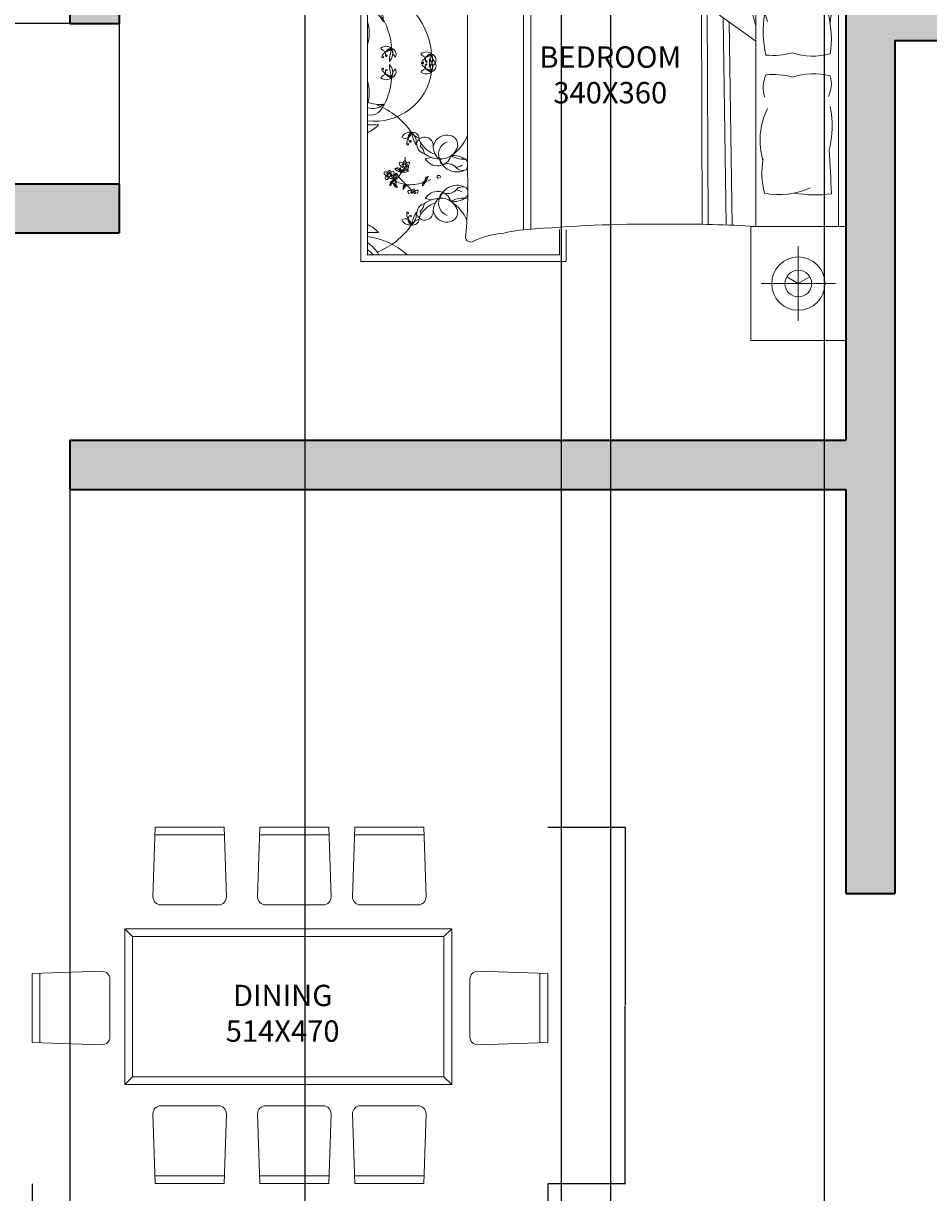
# Model space of a CAD drawing. Units: centimetres. Extents: x 2178 to 3635, y 1064 to 2635.
# Tile 6 of 9: x 2788 to 3211, y 1765 to 2312. Entities that reach past the tile are written whole.
import ezdxf

# ---------------------------------------------------------------- set-up
doc = ezdxf.new("R2010")
doc.units = ezdxf.units.CM
for name, color, linetype, lineweight in [('A-ANNO-DIMS', 2, 'Continuous', 18), ('A-AREA-IDEN', 7, 'Continuous', 18), ('A-DOOR', 32, 'Continuous', 25), ('A-FURN', 42, 'Continuous', 18), ('A-WALL', 7, 'Continuous', 35)]:
    doc.layers.add(name, color=color, linetype=linetype, lineweight=lineweight)
doc.layers.add('A-WALL-PATT', color=18, linetype='Continuous', lineweight=13, true_color=0x000000)
doc.styles.get("Standard").update_dxf_attribs({"font": 'arial.ttf'})
doc.dimstyles.get("Standard").update_dxf_attribs({"dimtxt": 0.18, "dimasz": 0.18, "dimexe": 0.18, "dimexo": 0.0625, "dimgap": 0.09, "dimtad": 0, "dimtih": 1, "dimtoh": 1, "dimdec": 4, "dimzin": 0, "dimdsep": 46, "dimtxsty": 'Standard', "dimcen": 0.09, "dimadec": 0, "dimazin": 0, "dimtfac": 1, "dimtdec": 4, "dimtofl": 0, "dimtmove": 0, "dimatfit": 3, "dimfxl": 1, "dimtolj": 1, "dimtzin": 0, "dimarcsym": 0})

# ---------------------------------------------------------------- blocks, each defined once
blk = doc.blocks.new('bed')
for p, q in [((2798.77, 2937.13), (3098.77, 2937.13)), ((2858.77, 2937.13), (2858.77, 2854.79)), ((2828.77, 2892.53), (2828.77, 2931.73)), ((3038.77, 2933.28), (2858.77, 2933.28)), ((3068.77, 2892.53), (3068.77, 2931.73)), ((2848.37, 2912.13), (2809.17, 2912.13)), ((3049.17, 2912.13), (3088.37, 2912.13)), ((2858.77, 2889.72), (3038.77, 2889.72)), ((2900.44, 2880.8), (2933.16, 2889.72)), ((2941.19, 2889.72), (2924.75, 2866.84)), ((2878.57, 2872.91), (2900.44, 2880.8)), ((2867.02, 2864.41), (2878.57, 2872.91)), ((3037.85, 2874.18), (2928.92, 2872.64)), ((3037.97, 2877.26), (2931.16, 2875.76)), ((2924.75, 2866.84), (2918.06, 2849.23)), ((2856.09, 2851.66), (2867.02, 2864.41)), ((3037.71, 2861.65), (2922.6, 2861.18)), ((3037.69, 2864.73), (2923.78, 2864.28)), ((2858.52, 2849.23), (2856.09, 2851.66)), ((2870.67, 2850.44), (2858.52, 2849.23)), ((2885.86, 2849.23), (2870.67, 2850.44)), ((2899.23, 2847.41), (2885.86, 2849.23)), ((2907.13, 2843.76), (2899.23, 2847.41)), ((2918.06, 2849.23), (2916.85, 2841.33)), ((2916.85, 2841.33), (2907.13, 2843.76)), ((2838.37, 2790.07), (2855.34, 2790.07)), ((2838.37, 2682), (2838.37, 2790.07)), ((2855.33, 2786.59), (2841.85, 2786.59)), ((2841.85, 2786.59), (2841.85, 2685.48)), ((3053.6, 2786.59), (3040.38, 2786.59)), ((3040.44, 2790.07), (3057.08, 2790.07)), ((3053.6, 2685.48), (3053.6, 2786.59)), ((3057.08, 2790.07), (3057.08, 2682)), ((3040.42, 2767.62), (2855.31, 2767.62)), ((3040.13, 2771.36), (2855.32, 2771.36)), ((3009.67, 2738.15), (2887.87, 2738.15)), ((2871.41, 2715.89), (2870.75, 2719.28)), ((2892.38, 2715.89), (2893.04, 2719.28)), ((3003.07, 2715.89), (3002.41, 2719.28)), ((3024.04, 2715.89), (3024.7, 2719.28)), ((3057.08, 2682), (2838.37, 2682)), ((2841.85, 2685.48), (3053.6, 2685.48))]:
    blk.add_line(p, q)
for points in [[(2858.77, 2887.13), (2798.77, 2887.13), (2798.77, 2937.13)], [(3038.77, 2937.13), (3038.77, 2887.13), (3098.77, 2887.13), (3098.77, 2937.13)], [(2828.77, 2912.13), (2832.27, 2918.19)], [(3068.77, 2912.13), (3065.27, 2918.19)], [(2828.77, 2912.13), (2832.27, 2906.07)], [(3068.77, 2912.13), (3065.27, 2906.07)]]:
    blk.add_lwpolyline(points)
for points in [[(2876, 2929.65, 0.074897), (2876.37, 2910.06, -0.472817)], [(2947.37, 2908.96, 0.14099), (2947.97, 2928.95, 0.235245)], [(2960.18, 2908.96, -0.14099), (2959.58, 2928.95, -0.235245)], [(3021.54, 2929.65, -0.074897), (3021.18, 2910.06, 0.472817)], [(2855.46, 2824.19, 0.001242), (2855.31, 2767.26, -0.127202), (2849.3, 2738.9)], [(3040.05, 2773.72, 0.056112), (3042.23, 2757.21, 0.095341), (3046.45, 2741.32)]]:
    blk.add_lwpolyline(points, format="xyb")
for centre, radius in [((2828.77, 2912.13), 14), ((3068.77, 2912.13), 14), ((2828.77, 2912.13), 7), ((3068.77, 2912.13), 7), ((2888.74, 2705.02), 0.764), ((3006.71, 2705.02), 0.764), ((2883.74, 2696.97), 0.764), ((3011.71, 2696.97), 0.764)]:
    blk.add_circle(centre, radius)
for centre, radius, start, end in [((3041.36, 5784.66), 2859.79, 266.68521, 267.14978), ((2917.11, 2821.09), 108.8, 82.21958, 99.49698), ((2940.09, 2876.08), 53.46, 81.52493, 103.95996), ((2963.69, 2914.69), 14.84, 63.34374, 106.10256), ((2985.93, 2877.16), 52.74, 76.34271, 101.1841), ((2856.18, 5784.66), 2859.79, 272.85022, 273.31479), ((2914.22, 2902.19), 38.67, 155.1316, 191.75834), ((2983.32, 2902.19), 38.67, 348.24166, 24.8684), ((2912, 2898.93), 36.76, 354.01289, 15.82928), ((2995.54, 2898.93), 36.76, 164.17072, 185.98711), ((2886.7, 2933.16), 40.2, 255.10393, 281.03689), ((2907.87, 2961.74), 69.73, 258.03974, 289.26152), ((2936.1, 2946.52), 52.9, 259.86169, 283.62376), ((2965.7, 2909.52), 15.9, 245.01826, 288.54073), ((2993.49, 2930.2), 38.19, 243.87611, 286.17464), ((3010.84, 2933.16), 40.2, 258.96311, 284.89607), ((3576.57, 2853.06), 539.05, 176.09997, 180.92818), ((2581.02, 2844.2), 275.17, 355.82941, 1.55305), ((2888.28, 2822.94), 24.42, 66.26158, 101.3392), ((2861.22, 2957.89), 113.22, 267.45188, 281.3392), ((2937.68, 2954.7), 116.34, 250.11942, 259.33829), ((2916.17, 2841.09), 0.724, 268.86235, 19.75363), ((3740.68, 2833.46), 703.17, 179.11454, 184.87351), ((2852.06, 2739.09), 2.77, 183.97998, 297.34124), ((2884.29, 2425.86), 312.3, 89.34325, 95.68869), ((2850.89, 2717.02), 22.71, 33.66712, 63.29966), ((2881.32, 2730.53), 11.57, 145.78505, 184.73037), ((2859.22, 2735.93), 12.43, 328.82178, 9.15542), ((2874.61, 2734.83), 3.61, 120.0293, 142.32497), ((2868.85, 2732.7), 9.56, 289.28218, 29.1751), ((2873.09, 2735.54), 4.49, 311.56531, 23.83541), ((2874.61, 2734.83), 3.61, 44.45169, 63.55801), ((2894.94, 2732.7), 9.56, 150.8249, 250.71782), ((2890.7, 2735.54), 4.49, 156.16459, 228.43469), ((2889.17, 2734.83), 3.61, 113.22901, 135.54831), ((2889.17, 2734.83), 3.61, 37.67503, 66.71436), ((2882.46, 2730.53), 11.57, 355.26963, 34.21495), ((2904.56, 2735.93), 12.43, 169.71335, 211.17822), ((2912.89, 2717.02), 22.71, 111.49413, 146.33288), ((2982.56, 2717.02), 22.71, 33.66712, 68.50587), ((3012.99, 2730.53), 11.57, 145.78505, 184.73037), ((2990.89, 2735.93), 12.43, 328.82178, 10.28665), ((3006.28, 2734.83), 3.61, 113.28564, 142.32497), ((3000.51, 2732.7), 9.56, 289.28218, 29.1751), ((3006.28, 2734.83), 3.61, 44.45169, 66.71436), ((3004.75, 2735.54), 4.49, 311.56531, 23.83541), ((3018.86, 2446.37), 291.92, 85.24024, 91.80351), ((3026.6, 2732.7), 9.56, 150.8249, 250.71782), ((3022.36, 2735.54), 4.49, 156.16459, 228.43469), ((3020.84, 2734.83), 3.61, 106.63434, 135.54831), ((3020.84, 2734.83), 3.61, 37.67503, 72.58143), ((3014.13, 2730.53), 11.57, 355.26963, 34.21495), ((3036.23, 2735.93), 12.43, 169.24899, 211.17822), ((3044.56, 2717.02), 22.71, 113.64533, 146.33288), ((3044.17, 2739.79), 2.73, 246.52186, 33.82642), ((2864.12, 2727.92), 5.07, 84.48557, 181.05378), ((2862.56, 2724.18), 9.02, 355.29334, 76.921), ((2880.15, 2727.58), 6.15, 131.56531, 195.14713), ((2867.4, 2730.97), 8.62, 7.43599, 29.91487), ((2883.64, 2727.58), 6.15, 344.85287, 48.43469), ((2896.38, 2730.97), 8.62, 150.08513, 172.56401), ((2901.22, 2724.18), 9.02, 103.079, 184.70666), ((2899.66, 2727.92), 5.07, 358.94622, 95.51443), ((2995.79, 2727.92), 5.07, 84.48557, 181.05378), ((2994.23, 2724.18), 9.02, 355.29334, 76.921), ((3011.81, 2727.58), 6.15, 131.56531, 195.14713), ((2999.07, 2730.97), 8.62, 7.43599, 29.91487), ((3015.3, 2727.58), 6.15, 344.85287, 48.43469), ((3028.05, 2730.97), 8.62, 150.08513, 172.56401), ((3032.89, 2724.18), 9.02, 103.079, 184.70666), ((3031.33, 2727.92), 5.07, 358.94622, 95.51443), ((2866.2, 2727.2), 7.17, 174.94485, 262.88575), ((2869.01, 2729.92), 6.96, 201.58187, 291.42215), ((2867.69, 2722.36), 7.46, 299.90854, 73.1337), ((2872.41, 2725.49), 1.86, 257.30406, 15.14713), ((2896.09, 2722.36), 7.46, 106.8663, 240.09146), ((2891.37, 2725.49), 1.86, 164.85287, 282.69594), ((2894.77, 2729.92), 6.96, 248.57785, 338.41813), ((2897.59, 2727.2), 7.17, 277.11425, 5.05515), ((2997.86, 2727.2), 7.17, 174.94485, 262.88575), ((3000.68, 2729.92), 6.96, 201.58187, 291.42215), ((2999.36, 2722.36), 7.46, 299.90854, 73.1337), ((3004.08, 2725.49), 1.86, 257.30406, 15.14713), ((3027.76, 2722.36), 7.46, 106.8663, 240.09146), ((3023.04, 2725.49), 1.86, 164.85287, 282.69594), ((3026.44, 2729.92), 6.96, 248.57785, 338.41813), ((3029.25, 2727.2), 7.17, 277.11425, 5.05515), ((2864.55, 2715.65), 4.5, 80.26398, 250.86884), ((2855.62, 2725.56), 14.16, 301.26137, 341.7045), ((2864.95, 2728.79), 8.71, 272.3591, 324.04014), ((2855.49, 2724.42), 16.1, 326.28828, 356.5076), ((2881.32, 2730.53), 11.57, 212.70113, 216.34448), ((2903.55, 2707.57), 24.85, 153.0032, 159.89408), ((2882.75, 2722.67), 0.578, 102.70507, 280.43845), ((2882.69, 2723.02), 0.94, 280.43845, 100.41356), ((2882.46, 2730.53), 11.57, 323.65552, 327.29887), ((2898.83, 2728.79), 8.71, 215.95986, 267.6409), ((2908.3, 2724.42), 16.1, 183.4924, 213.71172), ((2908.16, 2725.56), 14.16, 198.2955, 238.73863), ((2899.24, 2715.65), 4.5, 289.13116, 99.73602), ((2951.1, 2680.2), 39.18, 94.46233, 172.25504), ((2951.27, 2716.33), 4.34, 137.78732, 219.11446), ((2946.34, 2716.47), 3.27, 298.5391, 58.36268), ((2951.26, 2719.13), 3.2, 177.75849, 283.85198), ((2951.17, 2718.35), 3.25, 63.02737, 163.80375), ((2947.89, 2725.94), 6.69, 271.45846, 315.37266), ((2950.61, 2713.61), 6.19, 45.54113, 114.31008), ((2956.25, 2745.4), 27.41, 252.59304, 267.25817), ((2957.43, 2722.47), 9.91, 198.91595, 238.01098), ((2954.84, 2713.61), 6.19, 65.68992, 134.45887), ((2949.2, 2745.4), 27.41, 272.74183, 287.40696), ((2954.28, 2718.35), 3.25, 16.19625, 116.97263), ((2957.56, 2725.94), 6.69, 224.62734, 268.54154), ((2948.02, 2722.47), 9.91, 301.98902, 341.08405), ((2954.19, 2719.13), 3.2, 256.14802, 2.24151), ((2959.11, 2716.47), 3.27, 121.63732, 241.4609), ((2954.18, 2716.33), 4.34, 320.88554, 42.21268), ((2953.08, 2689.24), 30.32, 352.86355, 81.81966), ((2996.21, 2715.65), 4.5, 80.26398, 250.86884), ((2987.29, 2725.56), 14.16, 301.26137, 341.7045), ((2996.62, 2728.79), 8.71, 272.3591, 324.04014), ((2987.15, 2724.42), 16.1, 326.28828, 356.5076), ((3012.99, 2730.53), 11.57, 212.70113, 216.34448), ((3012.76, 2723.02), 0.94, 79.58644, 259.56155), ((3012.7, 2722.67), 0.578, 259.56155, 77.29493), ((2991.9, 2707.57), 24.85, 20.10592, 26.9968), ((3014.13, 2730.53), 11.57, 323.65552, 327.29887), ((3030.5, 2728.79), 8.71, 215.95986, 267.6409), ((3039.96, 2724.42), 16.1, 183.4924, 213.71172), ((3039.83, 2725.56), 14.16, 198.2955, 238.73863), ((3030.9, 2715.65), 4.5, 289.13116, 99.73602), ((2860.73, 2709.42), 3.25, 92.95159, 193.72796), ((2854.09, 2714.37), 6.69, 301.38267, 345.29688), ((2863.62, 2710.77), 2.76, 63.97555, 143.26805), ((2863.47, 2717), 5.62, 265.96902, 344.3045), ((2869.52, 2709.53), 5.99, 96.1662, 141.58255), ((2875.21, 2711.65), 0.59, 345.23556, 144.9248), ((2879.44, 2713.73), 1.58, 101.32561, 154.46214), ((2877.17, 2719.07), 4.74, 280.25878, 300.65599), ((2878.27, 2722.86), 8.46, 268.32639, 277.13024), ((2903.55, 2707.57), 24.85, 163.58418, 183.82768), ((2876.15, 2719.06), 4.82, 308.21012, 316.30712), ((2879.11, 2715.89), 1.44, 278.34322, 4.28685), ((2878.31, 2717.16), 2.51, 300.65599, 332.63414), ((2880.2, 2715.5), 0.611, 55.76575, 157.44165), ((2881.15, 2716.07), 0.611, 84.37838, 186.05427), ((2880.58, 2718.52), 2.51, 269.18588, 301.16403), ((2881.32, 2717.22), 1.44, 237.53317, 323.47681), ((2879.92, 2721.32), 4.82, 285.51291, 293.60991), ((2883.07, 2715.9), 1.58, 87.35788, 140.49441), ((2879.43, 2720.42), 4.74, 301.16403, 321.56124), ((2875.57, 2721.25), 8.46, 324.68979, 333.49364), ((2894.26, 2709.53), 5.99, 38.41745, 83.8338), ((2900.32, 2717), 5.62, 195.6955, 274.03098), ((2900.16, 2710.77), 2.76, 36.73195, 116.02445), ((2903.05, 2709.42), 3.25, 346.27204, 87.04841), ((2909.69, 2714.37), 6.69, 194.70312, 238.61733), ((2951.92, 2716.43), 0.424, 283.85198, 219.92454), ((2952.44, 2714.47), 0.487, 238.01098, 71.55918), ((2952.52, 2714.71), 0.236, 71.55918, 188.01668), ((2953.01, 2714.47), 0.487, 108.44082, 301.98902), ((2952.93, 2714.71), 0.236, 351.98332, 108.44082), ((2953.49, 2716.59), 0.255, 320.19092, 256.02088), ((2992.4, 2709.42), 3.25, 92.95159, 193.72796), ((2985.76, 2714.37), 6.69, 301.38267, 345.29688), ((2995.29, 2710.77), 2.76, 63.97555, 143.26805), ((2995.13, 2717), 5.62, 265.96902, 344.3045), ((3001.19, 2709.53), 5.99, 96.1662, 141.58255), ((3012.38, 2715.9), 1.58, 39.50559, 92.64212), ((3016.02, 2720.42), 4.74, 218.43876, 238.83597), ((3019.88, 2721.25), 8.46, 206.50636, 215.31021), ((3014.13, 2717.22), 1.44, 216.52319, 302.46683), ((3014.87, 2718.52), 2.51, 238.83597, 270.81412), ((3015.53, 2721.32), 4.82, 246.39009, 254.48709), ((3014.3, 2716.07), 0.611, 353.94573, 95.62162), ((3016.34, 2715.89), 1.44, 175.71315, 261.65678), ((3015.25, 2715.5), 0.611, 22.55835, 124.23425), ((3017.14, 2717.16), 2.51, 207.36586, 239.34401), ((2991.9, 2707.57), 24.85, 356.17232, 16.41582), ((3019.3, 2719.06), 4.82, 223.69288, 231.78988), ((3018.28, 2719.07), 4.74, 239.34401, 259.74122), ((3017.18, 2722.86), 8.46, 262.86976, 271.67361), ((3016.01, 2713.73), 1.58, 25.53786, 78.67439), ((3020.24, 2711.65), 0.59, 35.0752, 194.76444), ((3031.98, 2717), 5.62, 195.6955, 274.03098), ((3025.93, 2709.53), 5.99, 38.41745, 83.8338), ((3031.83, 2710.77), 2.76, 36.73195, 116.02445), ((3041.36, 2714.37), 6.69, 194.70312, 238.61733), ((3034.72, 2709.42), 3.25, 346.27204, 87.04841), ((2812.68, 2680.2), 39.18, 7.74496, 41.8856), ((2879.7, 2676.32), 39.18, 124.38655, 158.59079), ((2861.82, 2707.73), 4.34, 167.71153, 249.03868), ((2862.6, 2705.03), 6.19, 75.46535, 144.23429), ((2851.64, 2735.41), 27.41, 282.51726, 297.18239), ((2857.48, 2705.38), 3.27, 328.46331, 88.28689), ((2864.1, 2716.11), 9.91, 228.84017, 267.9352), ((2860.42, 2710.14), 3.2, 207.6827, 313.77619), ((2862.34, 2708.13), 0.424, 313.77619, 249.71835), ((2863.71, 2706.94), 0.236, 101.4834, 217.94089), ((2863.76, 2706.7), 0.487, 267.9352, 101.4834), ((2874.99, 2710.74), 1.27, 101.56373, 142.6358), ((2873.93, 2709.56), 0.764, 273.27684, 86.72316), ((2874.97, 2708.15), 1.26, 217.76209, 259.04026), ((2874.82, 2710.28), 0.73, 91.10805, 181.86747), ((2876.33, 2709.83), 2.32, 203.42757, 227.61037), ((2875.59, 2708.82), 1.58, 80.3487, 133.65382), ((2875.31, 2710.12), 1.25, 229.78892, 317.67915), ((2873.96, 2711.74), 1.84, 288.72627, 352.50315), ((2873.9, 2707.47), 1.78, 355.05304, 68.36176), ((2875.3, 2707.17), 2.5, 83.08516, 105.71709), ((2875.09, 2707.37), 0.586, 232.47371, 355.05304), ((2857.98, 2686.43), 28.48, 43.15413, 52.0459), ((2875.75, 2709.72), 0.658, 317.67915, 80.3487), ((2877.32, 2705.8), 1.44, 278.34322, 4.28685), ((2876.52, 2707.06), 2.51, 300.65599, 332.63414), ((2878.41, 2705.4), 0.611, 55.76575, 157.44165), ((2891.17, 2706.94), 12.46, 184.75602, 209.20408), ((2909.1, 2733.46), 40.99, 222.24124, 232.17444), ((2882.89, 2706.16), 3.48, 304.53686, 16.36991), ((2887.73, 2705.18), 2.46, 127.31045, 187.92519), ((2884.34, 2705.45), 2.53, 355.01064, 41.65801), ((2887.9, 2706.08), 1.04, 126.10456, 271.42811), ((2887.78, 2706.37), 0.749, 353.75256, 131.70535), ((2887.08, 2705.48), 1.05, 0.06451, 61.15075), ((2887.33, 2706.37), 1.2, 311.84125, 355.78771), ((2889.8, 2706.2), 1.27, 101.56373, 176.36503), ((2889.63, 2705.74), 0.73, 91.10805, 181.86747), ((2888.77, 2707.2), 1.84, 288.72627, 352.50315), ((2890.02, 2707.11), 0.59, 345.23556, 144.9248), ((2900.02, 2706.7), 0.487, 78.5166, 272.0648), ((2901.18, 2705.03), 6.19, 35.76571, 104.53465), ((2912.15, 2735.41), 27.41, 242.81761, 257.48274), ((2899.68, 2716.11), 9.91, 272.0648, 311.15983), ((2900.07, 2706.94), 0.236, 322.05911, 78.5166), ((2903.37, 2710.14), 3.2, 226.22381, 332.3173), ((2901.49, 2708.3), 0.255, 290.26671, 226.22708), ((2906.3, 2705.38), 3.27, 91.71311, 211.53669), ((2901.96, 2707.73), 4.34, 290.96132, 12.28847), ((2884.08, 2676.32), 39.18, 21.40921, 55.61345), ((3011.37, 2676.32), 39.18, 124.38655, 158.59079), ((2993.49, 2707.73), 4.34, 167.71153, 249.03868), ((2994.27, 2705.03), 6.19, 75.46535, 144.23429), ((2983.3, 2735.41), 27.41, 282.51726, 297.18239), ((2992.08, 2710.14), 3.2, 207.6827, 313.77619), ((2995.76, 2716.11), 9.91, 228.84017, 267.9352), ((2989.15, 2705.38), 3.27, 328.46331, 88.28689), ((2994.01, 2708.13), 0.424, 313.77619, 249.71835), ((2995.38, 2706.94), 0.236, 101.4834, 217.94089), ((2995.43, 2706.7), 0.487, 267.9352, 101.4834), ((3005.43, 2707.11), 0.59, 35.0752, 194.76444), ((3006.68, 2707.2), 1.84, 187.49685, 251.27373), ((3005.82, 2705.74), 0.73, 358.13253, 88.89195), ((3005.65, 2706.2), 1.27, 3.63497, 78.43627), ((3007.67, 2706.37), 0.749, 48.29465, 186.24744), ((3008.12, 2706.37), 1.2, 184.21229, 228.15875), ((3008.37, 2705.48), 1.05, 118.84925, 179.93549), ((3007.55, 2706.08), 1.04, 268.57189, 53.89544), ((3011.11, 2705.45), 2.53, 138.34199, 184.98936), ((3012.56, 2706.16), 3.48, 163.63009, 235.46314), ((3007.72, 2705.18), 2.46, 352.07481, 52.68955), ((2986.35, 2733.46), 40.99, 307.82556, 317.75876), ((3004.28, 2706.94), 12.46, 330.79592, 355.24398), ((3037.47, 2686.43), 28.48, 127.9541, 136.84587), ((3017.04, 2705.4), 0.611, 22.55835, 124.23425), ((3018.13, 2705.8), 1.44, 175.71315, 261.65678), ((3018.93, 2707.06), 2.51, 207.36586, 239.34401), ((3019.7, 2709.72), 0.658, 99.6513, 222.32085), ((3020.14, 2710.12), 1.25, 222.32085, 310.21108), ((3019.86, 2708.82), 1.58, 46.34618, 99.6513), ((3021.49, 2711.74), 1.84, 187.49685, 251.27373), ((3021.55, 2707.47), 1.78, 111.63824, 184.94696), ((3020.36, 2707.37), 0.586, 184.94696, 307.52629), ((3020.15, 2707.17), 2.5, 74.28291, 96.91484), ((3020.63, 2710.28), 0.73, 358.13253, 88.89195), ((3019.12, 2709.83), 2.32, 312.38963, 336.57243), ((3020.46, 2710.74), 1.27, 37.3642, 78.43627), ((3020.48, 2708.15), 1.26, 280.95974, 322.23791), ((3021.52, 2709.56), 0.764, 93.27684, 266.72316), ((3031.69, 2706.7), 0.487, 78.5166, 272.0648), ((3032.85, 2705.03), 6.19, 35.76571, 104.53465), ((3043.81, 2735.41), 27.41, 242.81761, 257.48274), ((3031.35, 2716.11), 9.91, 272.0648, 311.15983), ((3031.74, 2706.94), 0.236, 322.05911, 78.5166), ((3035.03, 2710.14), 3.2, 226.22381, 332.3173), ((3033.16, 2708.3), 0.255, 290.26671, 226.22708), ((3037.97, 2705.38), 3.27, 91.71311, 211.53669), ((3033.63, 2707.73), 4.34, 290.96132, 12.28847), ((3015.75, 2676.32), 39.18, 21.40921, 55.61345), ((3082.77, 2680.2), 39.18, 138.1144, 172.25504), ((2877.65, 2703.63), 1.58, 101.32561, 154.46214), ((2875.39, 2708.98), 4.74, 280.25878, 300.65599), ((2876.48, 2712.77), 8.46, 268.32639, 277.13024), ((2878.18, 2700.87), 0.853, 146.86359, 236.90213), ((2874.36, 2708.97), 4.82, 308.21012, 316.30712), ((2890.21, 2719.66), 22.32, 235.1882, 238.88441), ((2879.65, 2702.11), 2.31, 199.47987, 267.68284), ((2879.39, 2701.23), 1.99, 212.81548, 277.39917), ((2879.13, 2701.31), 0.883, 238.88441, 314.26458), ((2878.94, 2699.33), 1.99, 280.30568, 17.1958), ((2880.21, 2699.7), 0.666, 19.36054, 201.75478), ((2880.22, 2700.2), 0.666, 311.87034, 134.26458), ((2892.74, 2694.13), 13.31, 153.78194, 158.29129), ((2882.15, 2703.22), 3.48, 247.23048, 319.06353), ((2881, 2702.05), 2.05, 264.45436, 310.61881), ((2891.17, 2706.94), 12.46, 214.00334, 222.49171), ((2882.5, 2701.23), 2.12, 218.32082, 298.81623), ((2892.45, 2690.4), 14.94, 120.54402, 139.81798), ((2883.94, 2698.62), 2.46, 70.00407, 130.61881), ((2882.35, 2701.62), 2.53, 297.70426, 344.35163), ((2884.75, 2705.38), 2.12, 272.84988, 356.12261), ((2883.26, 2704.56), 2.05, 321.76073, 7.92519), ((2883.69, 2701.61), 2.05, 8.72271, 54.88717), ((2883.8, 2699.97), 3.48, 0.278, 72.11105), ((2885.36, 2701.25), 2.12, 20.5253, 88.5375), ((2888.15, 2702.29), 2.46, 188.72271, 249.33746), ((2887.13, 2703.59), 0.757, 148.0499, 225.62681), ((2892.45, 2690.4), 14.94, 113.05007, 113.84774), ((2888.54, 2702.71), 2.41, 104.75581, 148.0499), ((2887.18, 2704.44), 1.51, 247.40857, 351.43859), ((2884.99, 2701.06), 2.53, 334.9899, 21.63727), ((2887.61, 2704.38), 0.506, 262.90601, 7.13198), ((2889.78, 2703.61), 1.26, 151.21959, 259.04026), ((2891.14, 2705.29), 2.32, 203.42757, 227.61037), ((2890.41, 2704.28), 1.58, 80.3487, 133.65382), ((2890.12, 2705.58), 1.25, 229.78892, 317.67915), ((2888.71, 2702.93), 1.78, 355.05304, 68.36176), ((2890.11, 2702.63), 2.5, 83.08516, 105.71709), ((2889.9, 2702.83), 0.586, 232.47371, 355.05304), ((2890.56, 2705.18), 0.658, 317.67915, 80.3487), ((2892.45, 2690.4), 14.94, 87.10709, 94.75853), ((2948.18, 2697.36), 3.25, 63.02737, 163.80375), ((2944.89, 2704.96), 6.69, 271.45846, 315.37266), ((2957.27, 2697.36), 3.25, 16.19625, 116.97263), ((2960.56, 2704.96), 6.69, 224.62734, 268.54154), ((3003, 2690.4), 14.94, 85.24147, 92.89291), ((3004.89, 2705.18), 0.658, 99.6513, 222.32085), ((3005.33, 2705.58), 1.25, 222.32085, 310.21108), ((3005.04, 2704.28), 1.58, 46.34618, 99.6513), ((3006.74, 2702.93), 1.78, 111.63824, 184.94696), ((3005.55, 2702.83), 0.586, 184.94696, 307.52629), ((3005.34, 2702.63), 2.5, 74.28291, 96.91484), ((3004.31, 2705.29), 2.32, 312.38963, 336.57243), ((3005.67, 2703.61), 1.26, 280.95974, 28.78041), ((3008.27, 2704.44), 1.51, 188.56141, 292.59143), ((3007.84, 2704.38), 0.506, 172.86802, 277.09399), ((3006.91, 2702.71), 2.41, 31.9501, 75.24419), ((3010.46, 2701.06), 2.53, 158.36273, 205.0101), ((3010.09, 2701.25), 2.12, 91.4625, 159.4747), ((3011.65, 2699.97), 3.48, 107.88895, 179.722), ((3007.3, 2702.29), 2.46, 290.66254, 351.27729), ((3010.7, 2705.38), 2.12, 183.87739, 267.15012), ((3008.32, 2703.59), 0.757, 314.37319, 31.9501), ((3003, 2690.4), 14.94, 66.15226, 66.94993), ((3011.76, 2701.61), 2.05, 125.11283, 171.27729), ((3012.19, 2704.56), 2.05, 172.07481, 218.23927), ((3003, 2690.4), 14.94, 40.18202, 59.45598), ((3011.51, 2698.62), 2.46, 49.38119, 109.99593), ((3013.3, 2703.22), 3.48, 220.93647, 292.76952), ((3013.1, 2701.62), 2.53, 195.64837, 242.29574), ((3012.95, 2701.23), 2.12, 241.18377, 321.67918), ((3014.45, 2702.05), 2.05, 229.38119, 275.54564), ((3004.28, 2706.94), 12.46, 317.50829, 325.99666), ((3016.51, 2699.33), 1.99, 162.8042, 259.69432), ((3015.23, 2700.2), 0.666, 45.73542, 228.12966), ((3015.24, 2699.7), 0.666, 338.24522, 160.63946), ((3002.71, 2694.13), 13.31, 21.70871, 26.21806), ((3016.32, 2701.31), 0.883, 225.73542, 301.11559), ((3016.06, 2701.23), 1.99, 262.60083, 327.18452), ((3015.8, 2702.11), 2.31, 272.31716, 340.52013), ((3005.24, 2719.66), 22.32, 301.11559, 304.8118), ((3021.09, 2708.97), 4.82, 223.69288, 231.78988), ((3020.06, 2708.98), 4.74, 239.34401, 259.74122), ((3017.27, 2700.87), 0.853, 303.09787, 33.13641), ((3018.97, 2712.77), 8.46, 262.86976, 271.67361), ((3017.8, 2703.63), 1.58, 25.53786, 78.67439), ((2878.23, 2699.91), 2.31, 266.97007, 338.29129), ((2866.06, 2716.39), 22.32, 302.6784, 306.37461), ((2878.82, 2698.08), 0.853, 214.3538, 304.39233), ((2878.77, 2699.13), 0.883, 306.37461, 21.75478), ((2882.14, 2695.53), 0.757, 148.0499, 225.62681), ((2883.54, 2694.66), 2.41, 104.75581, 148.0499), ((2882.19, 2696.38), 1.51, 247.40857, 351.43859), ((2882.9, 2698.03), 1.04, 126.10456, 271.42811), ((2882.78, 2698.31), 0.749, 353.75256, 131.70535), ((2882.61, 2696.32), 0.506, 262.90601, 7.13198), ((2882.08, 2697.42), 1.05, 0.06451, 61.15075), ((2882.33, 2698.32), 1.2, 311.84125, 355.78771), ((2884.78, 2695.55), 1.26, 151.21959, 259.04026), ((2884.8, 2698.15), 1.27, 101.56373, 176.36503), ((2884.63, 2697.69), 0.73, 91.10805, 181.86747), ((2886.15, 2697.23), 2.32, 203.42757, 227.61037), ((2885.41, 2696.22), 1.58, 80.3487, 133.65382), ((2885.13, 2697.53), 1.25, 229.78892, 317.67915), ((2883.78, 2699.15), 1.84, 288.72627, 352.50315), ((2883.72, 2694.88), 1.78, 355.05304, 68.36176), ((2885.11, 2694.58), 2.5, 83.08516, 105.71709), ((2885.03, 2699.06), 0.59, 345.23556, 144.9248), ((2884.9, 2694.78), 0.586, 232.47371, 355.05304), ((2885.56, 2697.13), 0.658, 317.67915, 80.3487), ((2931.45, 2674.95), 19.09, 91.27197, 146.53828), ((2938.32, 2671.39), 23.79, 107.85038, 143.69643), ((2950.82, 2664.7), 35.39, 124.01234, 144.05304), ((2948.1, 2659.21), 39.18, 94.46233, 117.4146), ((2948.27, 2695.35), 4.34, 137.78732, 219.11446), ((2943.34, 2695.48), 3.27, 298.5391, 58.36268), ((2948.26, 2698.14), 3.2, 177.75849, 283.85198), ((2947.61, 2692.63), 6.19, 45.54113, 114.31008), ((2954.43, 2701.48), 9.91, 198.91595, 238.01098), ((2953.26, 2724.42), 27.41, 252.59304, 267.25817), ((2948.92, 2695.44), 0.424, 283.85198, 219.92454), ((2949.44, 2693.49), 0.487, 238.01098, 71.55918), ((2949.52, 2693.73), 0.236, 71.55918, 188.01668), ((2957.84, 2692.63), 6.19, 65.68992, 134.45887), ((2952.19, 2724.42), 27.41, 272.74183, 287.40696), ((2956.01, 2693.49), 0.487, 108.44082, 301.98902), ((2955.93, 2693.73), 0.236, 351.98332, 108.44082), ((2956.49, 2695.61), 0.255, 320.19092, 256.02088), ((2951.02, 2701.48), 9.91, 301.98902, 341.08405), ((2957.19, 2698.14), 3.2, 256.14802, 2.24151), ((2962.11, 2695.48), 3.27, 121.63732, 241.4609), ((2957.18, 2695.35), 4.34, 320.88554, 42.21268), ((2957.35, 2659.21), 39.18, 62.5854, 85.53767), ((2957, 2692.01), 17.54, 338.11703, 6.61954), ((2973.09, 2687.13), 7.03, 346.38982, 79.07385), ((2967.81, 2688.1), 8.89, 342.86088, 41.90487), ((3009.89, 2697.13), 0.658, 99.6513, 222.32085), ((3010.32, 2697.53), 1.25, 222.32085, 310.21108), ((3010.04, 2696.22), 1.58, 46.34618, 99.6513), ((3010.42, 2699.06), 0.59, 35.0752, 194.76444), ((3011.67, 2699.15), 1.84, 187.49685, 251.27373), ((3011.73, 2694.88), 1.78, 111.63824, 184.94696), ((3010.55, 2694.78), 0.586, 184.94696, 307.52629), ((3010.34, 2694.58), 2.5, 74.28291, 96.91484), ((3010.82, 2697.69), 0.73, 358.13253, 88.89195), ((3009.3, 2697.23), 2.32, 312.38963, 336.57243), ((3010.65, 2698.15), 1.27, 3.63497, 78.43627), ((3010.67, 2695.55), 1.26, 280.95974, 28.78041), ((3013.26, 2696.38), 1.51, 188.56141, 292.59143), ((3012.67, 2698.31), 0.749, 48.29465, 186.24744), ((3013.12, 2698.32), 1.2, 184.21229, 228.15875), ((3013.37, 2697.42), 1.05, 118.84925, 179.93549), ((3012.84, 2696.32), 0.506, 172.86802, 277.09399), ((3012.55, 2698.03), 1.04, 268.57189, 53.89544), ((3011.91, 2694.66), 2.41, 31.9501, 75.24419), ((3013.31, 2695.53), 0.757, 314.37319, 31.9501), ((3017.22, 2699.91), 2.31, 201.70871, 273.02993), ((3016.68, 2699.13), 0.883, 158.24522, 233.62539), ((3029.39, 2716.39), 22.32, 233.62539, 237.3216), ((3016.63, 2698.08), 0.853, 235.60767, 325.6462), ((2832.33, 2674.95), 19.09, 33.46172, 60.11157), ((2825.46, 2671.39), 23.79, 36.30357, 46.48142), ((2843.02, 2679.37), 15.93, 22.55474, 48.95456), ((2799.39, 2687.93), 54.2, 357.40811, 3.65191), ((2920.76, 2679.37), 15.93, 131.04544, 157.44526), ((2964.39, 2687.93), 54.2, 176.34809, 182.59189), ((2931.06, 2687.93), 54.2, 357.40811, 3.65191), ((2974.69, 2679.37), 15.93, 22.55474, 48.95456), ((3052.43, 2679.37), 15.93, 131.04544, 157.44526), ((3096.06, 2687.93), 54.2, 176.34809, 182.59189), ((3063.12, 2674.95), 19.09, 119.88843, 146.53828), ((3069.99, 2671.39), 23.79, 133.51858, 143.69643), ((2937.15, 2664.88), 21.54, 73.54311, 107.0202), ((2945.68, 2653.78), 31.85, 94.37872, 95.63574), ((2962.46, 2631.95), 56.92, 109.72171, 109.90284), ((2968.3, 2664.88), 21.54, 72.9798, 106.45689), ((2959.77, 2653.78), 31.85, 84.36426, 85.62128), ((2942.99, 2631.95), 56.92, 70.09716, 70.27829)]:
    blk.add_arc(centre, radius, start, end)
blk = doc.blocks.new('dt')
for p, q in [((2838.86, 1884.35), (2835.22, 1887.99)), ((2984.57, 1884.35), (2988.21, 1887.99)), ((2838.86, 1818.78), (2835.22, 1815.14)), ((2984.57, 1818.78), (2988.21, 1815.14))]:
    blk.add_line(p, q)
for points in [[(2882.82, 1902.95), (2881.73, 1935.61), (2849.55, 1935.61), (2848.46, 1902.95, 0.424007), (2852.1, 1899.18), (2879.18, 1899.18, 0.424007)], [(2931.78, 1902.95), (2930.69, 1935.61), (2898.51, 1935.61), (2897.42, 1902.95, 0.424007), (2901.06, 1899.18), (2928.14, 1899.18, 0.424007)], [(2976.19, 1902.95), (2975.1, 1935.61), (2942.92, 1935.61), (2941.83, 1902.95, 0.424007), (2945.47, 1899.18), (2972.55, 1899.18, 0.424007)], [(2824.57, 1833.77), (2791.91, 1834.86), (2791.91, 1867.04), (2824.57, 1868.12, -0.424007), (2828.33, 1864.48), (2828.33, 1837.41, -0.424007)], [(3000.5, 1833.77), (3033.17, 1834.86), (3033.17, 1867.04), (3000.5, 1868.12, 0.424007), (2996.74, 1864.48), (2996.74, 1837.41, 0.424007)], [(2882.82, 1801.45), (2881.73, 1768.79), (2849.55, 1768.79), (2848.46, 1801.45, -0.424007), (2852.1, 1805.22), (2879.18, 1805.22, -0.424007)], [(2931.78, 1801.45), (2930.69, 1768.79), (2898.51, 1768.79), (2897.42, 1801.45, -0.424007), (2901.06, 1805.22), (2928.14, 1805.22, -0.424007)], [(2976.19, 1801.45), (2975.1, 1768.79), (2942.92, 1768.79), (2941.83, 1801.45, -0.424007), (2945.47, 1805.22), (2972.55, 1805.22, -0.424007)]]:
    blk.add_lwpolyline(points, format="xyb", close=True)
for points in [[(2849.43, 1931.97), (2881.85, 1931.97)], [(2898.39, 1931.97), (2930.81, 1931.97)], [(2942.8, 1931.97), (2975.22, 1931.97)], [(2795.55, 1867.16), (2795.55, 1834.74)], [(3029.52, 1867.16), (3029.52, 1834.74)], [(2849.43, 1772.43), (2881.85, 1772.43)], [(2898.39, 1772.43), (2930.81, 1772.43)], [(2942.8, 1772.43), (2975.22, 1772.43)]]:
    blk.add_lwpolyline(points)
for points in [[(2835.22, 1887.99), (2835.22, 1815.14), (2988.21, 1815.14), (2988.21, 1887.99)], [(2838.86, 1884.35), (2838.86, 1818.78), (2984.57, 1818.78), (2984.57, 1884.35)]]:
    blk.add_lwpolyline(points, close=True)
blk = doc.blocks.new('DOOR-0750')
blk.add_line((0, 0), (75, 0))
blk = doc.blocks.new('*D40')
at = {"layer": 'A-ANNO-DIMS', "color": 0, "lineweight": -2, "transparency": 16777216}
for p, q in [((2791.91, 1768.73), (2791.91, 1732.42)), ((3033.17, 1768.73), (3033.17, 1732.42)), ((2792.09, 1732.6), (2911.51, 1732.6)), ((3032.99, 1732.6), (2913.56, 1732.6))]:
    blk.add_line(p, q, dxfattribs=at)
at = {"layer": 'A-ANNO-DIMS', "color": 0, "transparency": 16777216}
for points in [[(2792.09, 1732.63), (2792.09, 1732.57), (2791.91, 1732.6)], [(3032.99, 1732.63), (3032.99, 1732.57), (3033.17, 1732.6)]]:
    blk.add_solid(points, dxfattribs=at)
at = {"layer": 'Defpoints', "color": 0, "transparency": 16777216}
for p in [(2791.91, 1768.79), (3033.17, 1768.79), (3033.17, 1732.6)]:
    blk.add_point(p, dxfattribs=at)
at = {"layer": 'A-ANNO-DIMS', "color": 0, "transparency": 16777216, "insert": (2912.54, 1732.6), "char_height": 0.18, "attachment_point": 5}
blk.add_mtext('\\A1;DINING SET 241', dxfattribs=at)
blk = doc.blocks.new('*D41')
at = {"layer": 'A-ANNO-DIMS', "color": 0, "lineweight": -2, "transparency": 16777216}
for p, q in [((3033.23, 1935.61), (3069.54, 1935.61)), ((3069.36, 1935.43), (3069.36, 1852.38)), ((3069.36, 1768.97), (3069.36, 1852.02)), ((3033.23, 1768.79), (3069.54, 1768.79))]:
    blk.add_line(p, q, dxfattribs=at)
at = {"layer": 'A-ANNO-DIMS', "color": 0, "transparency": 16777216}
for points in [[(3069.33, 1935.43), (3069.39, 1935.43), (3069.36, 1935.61)], [(3069.33, 1768.97), (3069.39, 1768.97), (3069.36, 1768.79)]]:
    blk.add_solid(points, dxfattribs=at)
at = {"layer": 'Defpoints', "color": 0, "transparency": 16777216}
for p in [(3033.17, 1935.61), (3069.36, 1935.61), (3033.17, 1768.79)]:
    blk.add_point(p, dxfattribs=at)
at = {"layer": 'A-ANNO-DIMS', "color": 0, "transparency": 16777216, "insert": (3069.36, 1852.2), "char_height": 0.18, "attachment_point": 5}
blk.add_mtext('\\A1;167', dxfattribs=at)
blk = doc.blocks.new('*D61')
at = {"layer": 'A-ANNO-DIMS', "color": 0, "lineweight": -2, "transparency": 16777216}
for p, q in [((2919.6, 1623.65), (2919.6, 2634.77)), ((2919.78, 2634.59), (2979.32, 2634.59)), ((3039.42, 2634.59), (2979.88, 2634.59)), ((3039.6, 1623.65), (3039.6, 2634.77))]:
    blk.add_line(p, q, dxfattribs=at)
at = {"layer": 'A-ANNO-DIMS', "color": 0, "transparency": 16777216}
for points in [[(2919.78, 2634.62), (2919.78, 2634.56), (2919.6, 2634.59)], [(3039.42, 2634.62), (3039.42, 2634.56), (3039.6, 2634.59)]]:
    blk.add_solid(points, dxfattribs=at)
at = {"layer": 'Defpoints', "color": 0, "transparency": 16777216}
for p in [(3039.6, 2634.59), (2919.6, 1623.59), (3039.6, 1623.59)]:
    blk.add_point(p, dxfattribs=at)
at = {"layer": 'A-ANNO-DIMS', "color": 0, "transparency": 16777216, "insert": (2979.6, 2634.59), "char_height": 0.18, "attachment_point": 5}
blk.add_mtext('\\A1;120', dxfattribs=at)
blk = doc.blocks.new('*D62')
at = {"layer": 'A-ANNO-DIMS', "color": 0, "lineweight": -2, "transparency": 16777216}
for p, q in [((3062.6, 1623.65), (3062.6, 2634.77)), ((3062.78, 2634.59), (3112.32, 2634.59)), ((3162.42, 2634.59), (3112.88, 2634.59)), ((3162.6, 1623.65), (3162.6, 2634.77))]:
    blk.add_line(p, q, dxfattribs=at)
at = {"layer": 'A-ANNO-DIMS', "color": 0, "transparency": 16777216}
for points in [[(3062.78, 2634.62), (3062.78, 2634.56), (3062.6, 2634.59)], [(3162.42, 2634.62), (3162.42, 2634.56), (3162.6, 2634.59)]]:
    blk.add_solid(points, dxfattribs=at)
at = {"layer": 'Defpoints', "color": 0, "transparency": 16777216}
for p in [(3162.6, 2634.59), (3062.6, 1623.59), (3162.6, 1623.59)]:
    blk.add_point(p, dxfattribs=at)
at = {"layer": 'A-ANNO-DIMS', "color": 0, "transparency": 16777216, "insert": (3112.6, 2634.59), "char_height": 0.18, "attachment_point": 5}
blk.add_mtext('\\A1;100', dxfattribs=at)
blk = doc.blocks.new('*D63')
at = {"layer": 'A-ANNO-DIMS', "color": 0, "lineweight": -2, "transparency": 16777216}
for p, q in [((2699.6, 2093.53), (2699.6, 1113.41)), ((2809.6, 2093.53), (2809.6, 1113.41)), ((2699.78, 1113.59), (2754.32, 1113.59)), ((2809.42, 1113.59), (2754.88, 1113.59))]:
    blk.add_line(p, q, dxfattribs=at)
at = {"layer": 'A-ANNO-DIMS', "color": 0, "transparency": 16777216}
for points in [[(2699.78, 1113.62), (2699.78, 1113.56), (2699.6, 1113.59)], [(2809.42, 1113.62), (2809.42, 1113.56), (2809.6, 1113.59)]]:
    blk.add_solid(points, dxfattribs=at)
at = {"layer": 'Defpoints', "color": 0, "transparency": 16777216}
for p in [(2699.6, 2093.59), (2809.6, 2093.59), (2809.6, 1113.59)]:
    blk.add_point(p, dxfattribs=at)
at = {"layer": 'A-ANNO-DIMS', "color": 0, "transparency": 16777216, "insert": (2754.6, 1113.59), "char_height": 0.18, "attachment_point": 5}
blk.add_mtext('\\A1;110', dxfattribs=at)
blk = doc.blocks.new('*D66')
at = {"layer": 'A-ANNO-DIMS', "color": 0, "lineweight": -2, "transparency": 16777216}
for p, q in [((2832.54, 2311.59), (2757.42, 2311.59)), ((2757.6, 2311.41), (2757.6, 2274.27)), ((2757.6, 2236.77), (2757.6, 2273.91)), ((2832.54, 2236.59), (2757.42, 2236.59))]:
    blk.add_line(p, q, dxfattribs=at)
at = {"layer": 'A-ANNO-DIMS', "color": 0, "transparency": 16777216}
for points in [[(2757.57, 2311.41), (2757.63, 2311.41), (2757.6, 2311.59)], [(2757.57, 2236.77), (2757.63, 2236.77), (2757.6, 2236.59)]]:
    blk.add_solid(points, dxfattribs=at)
at = {"layer": 'Defpoints', "color": 0, "transparency": 16777216}
for p in [(2757.6, 2311.59), (2832.6, 2311.59), (2832.6, 2236.59)]:
    blk.add_point(p, dxfattribs=at)
at = {"layer": 'A-ANNO-DIMS', "color": 0, "transparency": 16777216, "insert": (2757.6, 2274.09), "char_height": 0.18, "attachment_point": 5}
blk.add_mtext('\\A1;75', dxfattribs=at)

msp = doc.modelspace()

# ---------------------------------------------------------------- hatches: boundary and pattern name
at = {"layer": 'A-WALL-PATT'}
h = msp.add_hatch(color=256, dxfattribs=at)
h.dxf.hatch_style = 1
h.paths.add_polyline_path([(2276.605, 2499.59), (2253.605, 2499.59), (2253.605, 2476.59), (2276.605, 2476.59)])
h.paths.add_polyline_path([(2411.605, 2350.59), (2253.605, 2350.59), (2253.605, 2327.59), (2411.605, 2327.59)])
h.paths.add_polyline_path([(2276.605, 2252.59), (2253.605, 2252.59), (2253.605, 2020.59), (2276.605, 2020.59), (2276.605, 2093.59), (2561.605, 2093.59), (2561.605, 2116.59), (2276.605, 2116.59)])
h.paths.add_polyline_path([(2659.605, 1787.59), (2610.616, 1787.59), (2276.605, 1787.59), (2276.605, 1860.59), (2253.605, 1860.59), (2253.605, 1732.09), (2276.605, 1732.09), (2276.605, 1764.59), (2516.605, 1764.59), (2516.605, 1699.59), (2539.605, 1699.59), (2539.605, 1764.59), (2659.605, 1764.59)])
h.paths.add_polyline_path([(2539.605, 1624.59), (2276.605, 1624.59), (2276.605, 1657.09), (2253.605, 1657.09), (2253.605, 1561.59), (2276.605, 1561.59), (2276.605, 1601.59), (2539.605, 1601.59)])
h.paths.add_polyline_path([(2276.605, 1501.59), (2253.605, 1501.59), (2253.605, 1371.59), (2276.605, 1371.59)])
h.paths.add_polyline_path([(2376.605, 1271.59), (2276.605, 1271.59), (2276.605, 1311.59), (2253.605, 1311.59), (2253.605, 1248.59), (2376.605, 1248.59)])
h.paths.add_polyline_path([(2636.605, 1271.59), (2536.605, 1271.59), (2536.605, 1248.59), (2636.605, 1248.59)])
h.paths.add_polyline_path([(2659.605, 1600.59), (2919.605, 1600.59), (2919.605, 1623.59), (2636.605, 1623.59), (2636.605, 1188.59), (2659.605, 1188.59)])
h.paths.add_polyline_path([(2939.605, 1211.59), (2759.605, 1211.59), (2759.605, 1188.59), (2939.605, 1188.59)])
h.paths.add_polyline_path([(3062.605, 1288.59), (3039.605, 1288.59), (3039.605, 1188.59), (3062.605, 1188.59)])
h.paths.add_polyline_path([(3372.605, 1248.59), (3062.605, 1248.59), (3062.605, 1218.59), (3372.605, 1218.59)])
h.paths.add_polyline_path([(3395.605, 1271.59), (3372.605, 1271.59), (3372.605, 1248.59), (3395.605, 1248.59)])
h.paths.add_polyline_path([(3559.605, 1271.59), (3536.605, 1271.59), (3536.605, 1248.59), (3559.605, 1248.59)])
h.paths.add_polyline_path([(3559.605, 1623.59), (3536.605, 1623.59), (3536.605, 1600.59), (3559.605, 1600.59)])
h.paths.add_polyline_path([(3395.605, 1623.59), (3162.605, 1623.59), (3162.605, 1600.59), (3395.605, 1600.59)])
h.paths.add_polyline_path([(3395.605, 1411.59), (3277.1, 1411.59), (3277.1, 1388.59), (3395.605, 1388.59)])
h.paths.add_polyline_path([(3157.1, 1411.59), (3062.605, 1411.59), (3062.605, 1623.59), (3039.605, 1623.59), (3039.605, 1388.59), (3157.1, 1388.59)])
h.paths.add_polyline_path([(3559.605, 1797.09), (3536.605, 1797.09), (3536.605, 1764.59), (3316.605, 1764.59), (3316.605, 1927.59), (3293.605, 1927.59), (3293.605, 1741.59), (3372.605, 1741.59), (3395.605, 1741.59), (3559.605, 1741.59)])
h.paths.add_polyline_path([(3559.605, 1990.59), (3536.605, 1990.59), (3536.605, 1974.446), (3536.605, 1927.59), (3391.605, 1927.59), (3391.605, 1904.59), (3536.605, 1904.59), (3536.605, 1872.09), (3559.605, 1872.09)])
h.paths.add_polyline_path([(3559.605, 2180.59), (3536.605, 2180.59), (3536.605, 2050.59), (3559.605, 2050.59)])
h.paths.add_polyline_path([(3559.605, 2326.59), (3446.105, 2326.59), (3446.105, 2303.59), (3536.605, 2303.59), (3536.605, 2240.59), (3559.605, 2240.59)])
h.paths.add_polyline_path([(3286.105, 2326.59), (3195.605, 2326.59), (3195.605, 2499.59), (3082.605, 2499.59), (3082.605, 2476.59), (3172.605, 2476.59), (3172.605, 2116.59), (2809.605, 2116.59), (2809.605, 2093.59), (3172.605, 2093.59), (3172.605, 1904.59), (3195.605, 1904.59), (3195.605, 2303.59), (3286.105, 2303.59)])
h.paths.add_polyline_path([(2832.605, 2236.59), (2659.605, 2236.59), (2659.605, 2476.59), (2697.105, 2476.59), (2697.105, 2499.59), (2636.605, 2499.59), (2636.605, 2093.59), (2699.605, 2093.59), (2699.605, 2116.59), (2659.605, 2116.59), (2659.605, 2213.59), (2832.605, 2213.59)])
h.paths.add_polyline_path([(2832.605, 2476.59), (2922.605, 2476.59), (2922.605, 2499.59), (2772.105, 2499.59), (2772.105, 2476.59), (2809.605, 2476.59), (2809.605, 2311.59), (2832.605, 2311.59)])

# ---------------------------------------------------------------- linework, layer by layer
at = {"layer": 'A-WALL'}
for p, q in [((2809.605, 2476.59), (2809.605, 2311.59)), ((2832.605, 2476.59), (2832.605, 2311.59)), ((3172.605, 2476.59), (3172.605, 2116.59)), ((2809.605, 2311.59), (2832.605, 2311.59)), ((3195.605, 2303.59), (3536.605, 2303.59)), ((3195.605, 2303.59), (3195.605, 1904.59)), ((2659.605, 2236.59), (2832.605, 2236.59)), ((2832.605, 2236.59), (2832.605, 2213.59)), ((2659.605, 2213.59), (2832.605, 2213.59)), ((2809.605, 2116.59), (3172.605, 2116.59)), ((2809.605, 2116.59), (2809.605, 2093.59)), ((2809.605, 2093.59), (3172.605, 2093.59)), ((3172.605, 2093.59), (3172.605, 1904.59)), ((3172.605, 1904.59), (3195.605, 1904.59))]:
    msp.add_line(p, q, dxfattribs=at)

# ---------------------------------------------------------------- block references
at = {"layer": 'A-DOOR', "rotation": 270.0000000000007}
msp.add_blockref('DOOR-0750', (2832.605, 2311.59), dxfattribs=at)
at = {"layer": 'A-FURN', "xscale": 0.8894661318613604, "yscale": 0.8894661318613604, "zscale": 0.8894661318613604, "rotation": 270}
msp.add_blockref('bed', (560.128, 4919.422), dxfattribs=at)
at = {"layer": 'A-FURN'}
msp.add_blockref('dt', (0, 0), dxfattribs=at)

# ---------------------------------------------------------------- texts
at = {"layer": 'A-AREA-IDEN', "char_height": 10, "attachment_point": 1}
for s, insert in [('\\pxqc;BEDROOM\\P340X360', (3006.625, 2300.829)), ('\\pxqc;DINING\\P514X470', (2853.349, 1861.821))]:
    msp.add_mtext_dynamic_manual_height_columns(s, width=111.5542, gutter_width=12.5, heights=[0], dxfattribs=dict(at, insert=insert))

# ---------------------------------------------------------------- dimensions: what is measured, and where the dimension line sits
at = {"layer": 'A-ANNO-DIMS'}
for base, p1, p2, picture, middle in [((3039.605, 2634.59), (2919.605, 1623.59), (3039.605, 1623.59), '*D61', (2979.605, 2634.59)), ((3162.605, 2634.59), (3062.605, 1623.59), (3162.605, 1623.59), '*D62', (3112.605, 2634.59)), ((2809.605, 1113.59), (2699.605, 2093.59), (2809.605, 2093.59), '*D63', (2754.605, 1113.59))]:
    dim = msp.add_linear_dim(base=base, p1=p1, p2=p2, dimstyle='Standard', override={"dimdec": 0, "dimlfac": 1, "dimrnd": 0, "dimzin": 0, "dimdsep": 46, "dimlunit": 2}, dxfattribs=at)
    dim.commit()
    dim.dimension.update_dxf_attribs({"geometry": picture, "text_midpoint": middle})
for base, p1, p2, picture, middle in [((2757.605, 2311.59), (2832.605, 2236.59), (2832.605, 2311.59), '*D66', (2757.605, 2274.09)), ((3069.356, 1935.61), (3033.166, 1768.791), (3033.166, 1935.61), '*D41', (3069.356, 1852.201))]:
    dim = msp.add_linear_dim(base=base, p1=p1, p2=p2, angle=90, dimstyle='Standard', override={"dimdec": 0, "dimlfac": 1, "dimrnd": 0, "dimzin": 0, "dimdsep": 46, "dimlunit": 2}, dxfattribs=at)
    dim.commit()
    dim.dimension.update_dxf_attribs({"geometry": picture, "text_midpoint": middle})
dim = msp.add_linear_dim(base=(3033.166, 1732.601), p1=(2791.905, 1768.791), p2=(3033.166, 1768.791), text='DINING SET <>', dimstyle='Standard', override={"dimdec": 0, "dimlfac": 1, "dimrnd": 0, "dimzin": 0, "dimdsep": 46, "dimlunit": 2}, dxfattribs=at)
dim.commit()
dim.dimension.update_dxf_attribs({"geometry": '*D40', "text_midpoint": (2912.536, 1732.601)})

doc.saveas('drawing.dxf')
